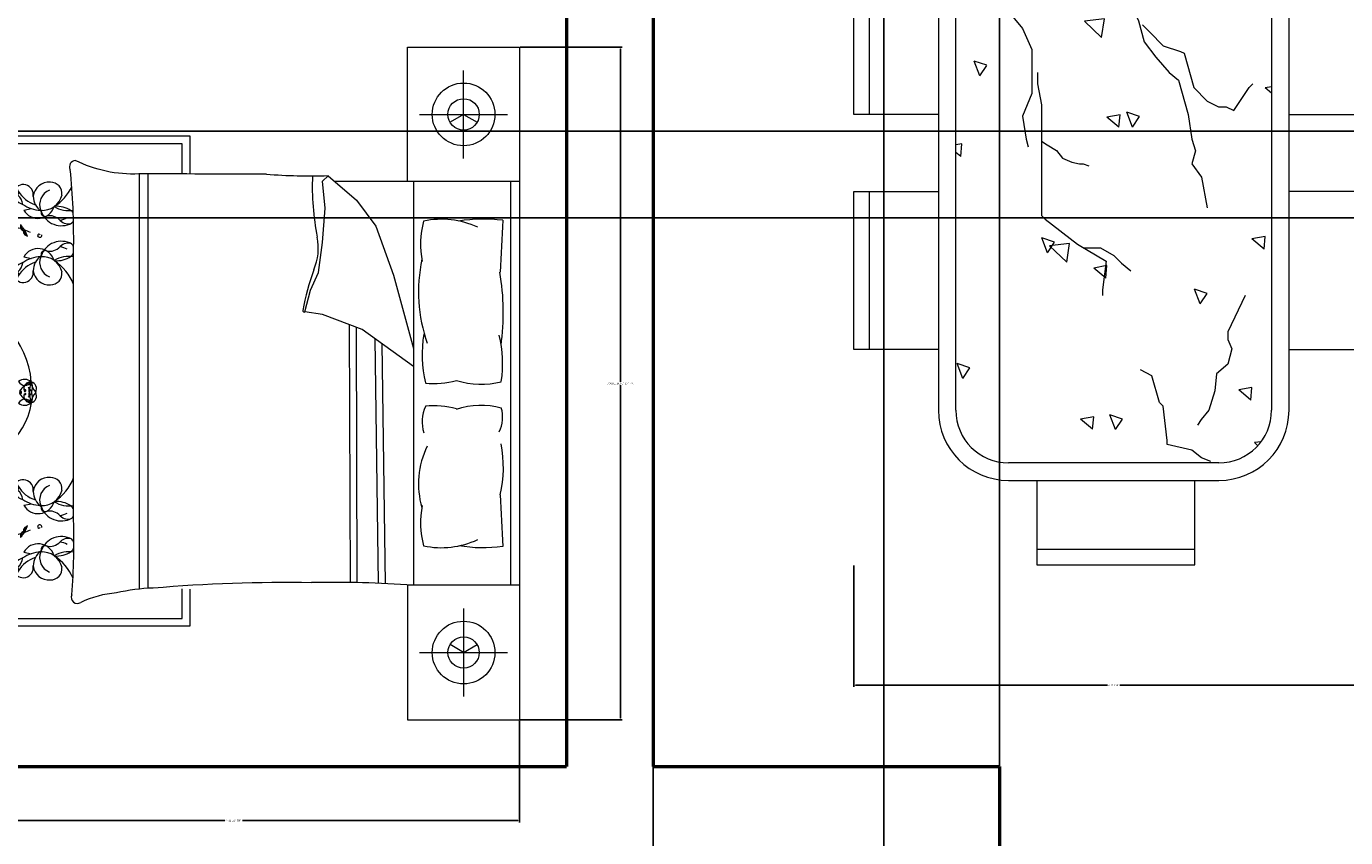
# Model space of a CAD drawing. Units: inches. Extents: x 3 to 576, y -689 to 51.
# Tile 7 of 21: x 199 to 336, y -514 to -429. Entities that reach past the tile are written whole.
import ezdxf

# ---------------------------------------------------------------- set-up
doc = ezdxf.new("R2010")
doc.units = ezdxf.units.IN
doc.header["$MEASUREMENT"] = 0
for name, color, linetype, lineweight in [('A-ANNO-DIMS', 2, 'Continuous', 18), ('A-FURN', 8, 'Continuous', 18), ('A-WALL', 7, 'Continuous', 50)]:
    doc.layers.add(name, color=color, linetype=linetype, lineweight=lineweight)
doc.styles.get("Standard").update_dxf_attribs({"font": 'arial.ttf'})
doc.dimstyles.get("Standard").update_dxf_attribs({"dimtxt": 0.18, "dimasz": 0.18, "dimexe": 0.18, "dimexo": 0.0625, "dimgap": 0.09, "dimtad": 0, "dimtih": 1, "dimtoh": 1, "dimdec": 0, "dimzin": 0, "dimdsep": 46, "dimlunit": 3, "dimtxsty": 'Standard', "dimcen": 0.09, "dimadec": 0, "dimazin": 0, "dimtfac": 1, "dimtdec": 0, "dimtofl": 0, "dimtmove": 0, "dimatfit": 3, "dimfxl": 1, "dimtolj": 1, "dimtzin": 0, "dimarcsym": 0})

# ---------------------------------------------------------------- blocks, each defined once
blk = doc.blocks.new('BED-DOUBLE')
for p, q in [((59.45, 69.91), (59.45, 0)), ((53.63, 58.35), (53.63, 67.49)), ((49.06, 62.92), (58.2, 62.92)), ((0, 60.68), (25.18, 60.68)), ((0, 9.72), (0, 60.68)), ((25.18, 60.68), (25.18, 56.73)), ((0.81, 59.87), (0.81, 10.53)), ((24.37, 59.87), (0.81, 59.87)), ((24.37, 56.73), (24.37, 59.87)), ((19.95, 13.6), (19.95, 56.73)), ((20.82, 13.66), (20.82, 56.73)), ((38.97, 55.99), (39.54, 56.55)), ((39.54, 56.55), (42.51, 54.01)), ((39.25, 53.16), (38.97, 55.99)), ((59.45, 55.93), (40.27, 55.93)), ((48.41, 55.93), (48.41, 13.98)), ((58.56, 13.98), (58.56, 55.93)), ((42.51, 54.01), (44.49, 51.31)), ((7.9, 52.98), (8.69, 53.14)), ((38.97, 49.62), (39.25, 53.16)), ((44.49, 51.31), (46.33, 46.22)), ((38.55, 46.5), (38.97, 49.62)), ((7.9, 48.1), (8.69, 47.94)), ((13.08, 20.76), (13.08, 49.15)), ((37.7, 44.66), (38.55, 46.5)), ((46.33, 46.22), (48.41, 38.59)), ((37.13, 42.39), (37.7, 44.66)), ((38.97, 42.11), (37.13, 42.39)), ((43.07, 40.55), (38.97, 42.11)), ((41.87, 14.23), (41.76, 41.05)), ((42.58, 14.23), (42.48, 40.78)), ((48.41, 36.72), (43.07, 40.55)), ((44.78, 14.2), (44.43, 39.58)), ((45.5, 14.17), (45.15, 39.06)), ((7.9, 22.3), (8.69, 22.46)), ((7.9, 17.41), (8.69, 17.26)), ((24.37, 10.53), (24.37, 13.61)), ((25.18, 13.59), (25.18, 9.72)), ((53.63, 11.56), (53.63, 2.42)), ((25.18, 9.72), (0, 9.72)), ((0.81, 10.53), (24.37, 10.53)), ((49.06, 6.99), (58.2, 6.99))]:
    blk.add_line(p, q)
for points in [[(47.8, 55.93), (47.8, 69.91), (59.45, 69.91)], [(53.63, 62.92), (52.22, 62.1)], [(53.63, 62.92), (55.04, 62.1)], [(59.45, 13.98), (47.8, 13.98), (47.8, 0), (59.45, 0)], [(53.63, 6.99), (52.22, 7.81)], [(53.63, 6.99), (55.04, 7.81)]]:
    blk.add_lwpolyline(points)
for points in [[(33.13, 56.7, 0.001242), (19.87, 56.73, -0.127202), (13.26, 58.14)], [(57.71, 51.91, 0.074897), (53.14, 51.83, -0.472817)], [(52.89, 35.28, 0.14099), (57.55, 35.14, 0.235245)], [(52.89, 32.3, -0.14099), (57.55, 32.44, -0.235245)], [(57.71, 18, -0.074897), (53.14, 18.08, 0.472817)], [(21.37, 13.68, 0.056112), (17.53, 13.18, 0.095341), (13.82, 12.19)]]:
    blk.add_lwpolyline(points, format="xyb")
for centre, radius in [((53.63, 62.92), 3.26), ((53.63, 62.92), 1.63), ((3.49, 50.11), 0.178), ((5.36, 48.94), 0.178), ((5.36, 21.45), 0.178), ((3.49, 20.29), 0.178), ((53.63, 6.99), 3.26), ((53.63, 6.99), 1.63)]:
    blk.add_circle(centre, radius)
for centre, radius, start, end in [((-2.47, 63.69), 5.54, 306.3036, 316.4814), ((-1.64, 62.09), 4.45, 303.4617, 330.1116), ((-0.42, 66.67), 9.13, 277.745, 311.8856), ((-1.32, 51.05), 9.13, 34.3865, 68.5908), ((13.3, 57.49), 0.645, 93.98, 207.3412), ((-0.61, 59.6), 3.71, 292.5547, 318.9546), ((1.38, 69.77), 12.63, 267.4081, 273.6519), ((-59.69, 49.98), 72.78, 359.3433, 5.6887), ((37.8, 120.65), 64.12, 265.8294, 271.553), ((64.29, 55.36), 26.39, 177.4519, 191.3392), ((6, 55.22), 1.01, 77.7115, 159.0387), ((5.45, 56.23), 0.762, 238.4633, 358.2869), ((7.95, 54.69), 2.31, 138.8402, 177.9352), ((6.56, 55.55), 0.747, 117.6827, 223.7762), ((6.09, 55.1), 0.0988, 223.7762, 159.7183), ((6.39, 55.47), 0.757, 2.9516, 103.728), ((12.45, 57.59), 6.39, 192.5173, 207.1824), ((5.37, 55.04), 1.44, 345.4653, 54.2343), ((7.54, 57.02), 1.56, 211.3827, 255.2969), ((7.84, 54.58), 1.05, 350.264, 160.8688), ((8.16, 54.83), 1.31, 175.969, 254.3045), ((6.7, 54.8), 0.643, 333.9755, 53.2681), ((10.15, 56.66), 3.3, 211.2614, 251.7045), ((10.53, 54.2), 1.67, 84.9449, 172.8857), ((11.17, 53.54), 1.62, 111.5819, 201.4221), ((10.7, 54.68), 1.18, 354.4856, 91.0538), ((8.16, 57.76), 5.29, 303.6671, 333.2997), ((5.76, 54.77), 0.113, 177.9352, 11.4834), ((5.81, 54.78), 0.0551, 11.4834, 127.9409), ((6.41, 53.42), 1.4, 6.1662, 51.5825), ((9.88, 56.69), 3.75, 236.2883, 266.5076), ((10.9, 54.49), 2.03, 182.3591, 234.0401), ((9.83, 55.04), 2.1, 265.2933, 346.921), ((5.91, 52.13), 0.137, 142.4737, 265.053), ((6.09, 52.15), 0.294, 127.7621, 169.0403), ((5.94, 52.4), 0.414, 265.053, 338.3618), ((6.48, 51.84), 0.541, 113.4276, 137.6104), ((6.42, 52.4), 0.178, 183.2768, 356.7232), ((6.55, 52.07), 0.291, 139.7889, 227.6792), ((5.87, 52.08), 0.583, 353.0852, 15.7171), ((6.25, 52.01), 0.368, 350.3487, 43.6538), ((6.93, 52.39), 0.428, 198.7263, 262.5032), ((6.59, 52.19), 0.17, 1.1081, 91.8675), ((6.91, 52.1), 0.138, 255.2356, 54.9248), ((6.7, 52.15), 0.297, 11.5637, 52.6358), ((9.4, 53.85), 1.74, 209.9085, 343.1337), ((10.13, 52.75), 0.434, 167.3041, 285.1471), ((11.31, 50.67), 2.7, 122.7011, 126.3445), ((11.81, 53.58), 2.23, 199.2822, 299.1751), ((10.62, 50.95), 1.43, 41.5653, 105.1471), ((12.57, 55.82), 2.9, 238.8218, 279.1554), ((11.31, 50.67), 2.7, 55.785, 94.7304), ((11.41, 53.92), 2.01, 277.436, 299.9149), ((12.31, 52.24), 0.842, 30.0293, 52.325), ((3.75, 51.26), 0.199, 124.3538, 214.3923), ((4.04, 51.23), 0.464, 190.3057, 287.1958), ((4.17, 51.39), 0.538, 176.9701, 248.2913), ((8.01, 54.23), 5.2, 212.6784, 216.3746), ((3.99, 51.27), 0.206, 216.3746, 291.7548), ((5.81, 48.38), 2.9, 124.0033, 132.4917), ((2.83, 48.01), 3.1, 63.7819, 68.2913), ((4.48, 50.4), 0.493, 128.3208, 208.8162), ((4.48, 51.12), 0.464, 122.8155, 187.3992), ((4.12, 50.93), 0.155, 289.3605, 111.7548), ((4.24, 50.93), 0.155, 221.8703, 44.2646), ((4.94, 50.48), 0.812, 157.2305, 229.0635), ((4.69, 51.06), 0.538, 109.4799, 177.6828), ((4.67, 50.75), 0.478, 174.4544, 220.6188), ((4.4, 51.4), 0.199, 56.8636, 146.9021), ((4.5, 51.18), 0.206, 148.8844, 224.2646), ((8.78, 48.6), 5.2, 145.1882, 148.8844), ((5.81, 48.38), 2.9, 94.756, 119.2041), ((11.99, 44.2), 9.55, 132.2412, 142.1744), ((7.17, 51.8), 1.97, 178.3264, 187.1302), ((5.04, 51.53), 0.367, 11.3256, 64.4621), ((6.29, 52.06), 1.1, 190.2588, 210.656), ((5.55, 51.61), 0.336, 188.3432, 274.2869), ((5.84, 51.79), 0.586, 210.656, 242.6341), ((6.28, 52.3), 1.12, 218.2101, 226.3071), ((5.45, 51.35), 0.142, 325.7657, 67.4417), ((1.03, 56.11), 6.64, 313.1541, 322.0459), ((5.96, 45.49), 5.79, 73.5842, 93.8277), ((6.46, 51.97), 0.153, 227.6792, 350.3487), ((9.52, 51.39), 1.97, 178.3264, 187.1302), ((7.39, 51.11), 0.367, 11.3256, 64.4621), ((8.64, 51.64), 1.1, 190.2588, 210.656), ((7.9, 51.19), 0.336, 188.3432, 274.2869), ((8.19, 51.38), 0.586, 210.656, 242.6341), ((8.64, 51.88), 1.12, 218.2101, 226.3071), ((7.81, 50.93), 0.142, 325.7657, 67.4417), ((8.21, 50.67), 0.336, 147.5332, 233.4768), ((7.94, 50.71), 0.142, 354.3784, 96.0543), ((8.51, 50.85), 0.586, 179.1859, 211.164), ((5.96, 45.49), 5.79, 63.0032, 69.8941), ((12.48, 52.59), 1.05, 221.5653, 293.8354), ((12.31, 52.24), 0.842, 314.4517, 333.558), ((58.53, 49.42), 9.37, 165.1039, 191.0369), ((51.31, 43.01), 9.01, 65.1316, 101.7583), ((723.03, 13.38), 666.43, 176.68521, 177.14978), ((2.98, 49.84), 0.137, 142.4737, 265.053), ((3.16, 49.87), 0.294, 61.2196, 169.0403), ((3, 50.12), 0.414, 265.053, 338.3618), ((3.35, 50.47), 0.351, 157.4086, 261.4386), ((3.15, 50.48), 0.176, 58.0499, 135.6268), ((3.55, 49.55), 0.541, 113.4276, 137.6104), ((3.34, 50.37), 0.118, 172.906, 277.132), ((2.95, 50.16), 0.561, 14.7558, 58.0499), ((3.62, 49.79), 0.291, 139.7889, 227.6792), ((3.53, 49.68), 0.153, 227.6792, 350.3487), ((3.74, 50.31), 0.243, 36.1046, 181.4281), ((2.93, 49.79), 0.583, 353.0852, 15.7171), ((3.31, 49.72), 0.368, 350.3487, 43.6538), ((3.59, 50.5), 0.245, 270.0645, 331.1507), ((3.8, 50.44), 0.28, 221.8413, 265.7877), ((4, 50.1), 0.428, 198.7263, 262.5032), ((3.66, 49.9), 0.17, 1.1081, 91.8675), ((3.8, 50.33), 0.174, 263.7526, 41.7054), ((3.76, 49.86), 0.297, 11.5637, 86.365), ((3.98, 49.81), 0.138, 255.2356, 54.9248), ((4.57, 50.43), 0.59, 207.7043, 254.3516), ((4.19, 50.1), 0.812, 270.278, 342.111), ((4.73, 49.08), 0.574, 98.7227, 159.3375), ((1.96, 48.08), 3.48, 30.544, 49.818), ((3.87, 50.06), 0.574, 340.0041, 40.6188), ((4.57, 50.12), 0.478, 278.7227, 324.8872), ((4.49, 49.73), 0.493, 290.5253, 358.5375), ((5.23, 49.31), 0.351, 157.4086, 261.4386), ((5.03, 49.32), 0.176, 58.0499, 135.6268), ((5.45, 49.87), 0.493, 182.8499, 266.1226), ((5.26, 50.22), 0.478, 231.7607, 277.9252), ((5.63, 50.31), 0.812, 214.5369, 286.3699), ((4.83, 48.99), 0.561, 14.7558, 58.0499), ((1.96, 48.08), 3.48, 23.0501, 23.8477), ((5.4, 49.18), 0.574, 37.3105, 97.9252), ((5.61, 49.14), 0.243, 36.1046, 181.4281), ((5.47, 49.97), 0.59, 265.0106, 311.658), ((8.95, 51.12), 1.1, 211.164, 231.5612), ((9.15, 52.01), 1.97, 234.6898, 243.4936), ((9.16, 51), 1.12, 195.5129, 203.6099), ((7.9, 50.27), 0.367, 357.3579, 50.4944), ((9.48, 50.34), 0.135, 12.7051, 190.4384), ((9.56, 50.36), 0.219, 190.4384, 10.4136), ((11.81, 47.5), 2.23, 60.8249, 160.7178), ((12.48, 48.49), 1.05, 66.1646, 138.4347), ((12.31, 48.84), 0.842, 23.229, 45.5483), ((32.84, 49.05), 5.69, 336.2616, 11.3392), ((4.44, 49.82), 0.59, 244.9899, 291.6373), ((4.85, 48.67), 0.137, 142.4737, 265.053), ((5.03, 48.7), 0.294, 61.2196, 169.0403), ((4.88, 48.95), 0.414, 265.053, 338.3618), ((5.43, 48.38), 0.541, 113.4276, 137.6104), ((5.21, 49.21), 0.118, 172.906, 277.132), ((5.5, 48.62), 0.291, 139.7889, 227.6792), ((5.4, 48.52), 0.153, 227.6792, 350.3487), ((4.81, 48.63), 0.583, 353.0852, 15.7171), ((1.96, 48.08), 3.48, 357.1071, 4.7585), ((5.19, 48.56), 0.368, 350.3487, 43.6538), ((5.47, 49.33), 0.245, 270.0645, 331.1507), ((5.68, 49.27), 0.28, 221.8413, 265.7877), ((5.87, 48.94), 0.428, 198.7263, 262.5032), ((5.53, 48.74), 0.17, 1.1081, 91.8675), ((5.68, 49.17), 0.174, 263.7526, 41.7054), ((5.64, 48.7), 0.297, 11.5637, 86.365), ((5.85, 48.65), 0.138, 255.2356, 54.9248), ((9.88, 44.39), 3.75, 93.4924, 123.7117), ((9.4, 47.23), 1.74, 16.8663, 150.0915), ((10.9, 46.59), 2.03, 125.9599, 177.6409), ((11.17, 47.54), 1.62, 158.5779, 248.4181), ((9.83, 46.04), 2.1, 13.079, 94.7067), ((10.13, 48.33), 0.434, 74.8529, 192.6959), ((11.31, 50.41), 2.7, 233.6555, 237.2989), ((10.62, 50.13), 1.43, 254.8529, 318.4347), ((12.57, 45.26), 2.9, 79.7133, 121.1782), ((11.31, 50.41), 2.7, 265.2696, 304.215), ((11.41, 47.16), 2.01, 60.0851, 82.564), ((12.31, 48.84), 0.842, 307.675, 336.7144), ((8.16, 46.25), 1.31, 105.6955, 184.031), ((7.84, 46.5), 1.05, 199.1312, 9.736), ((6.41, 47.66), 1.4, 308.4175, 353.8338), ((10.15, 44.42), 3.3, 108.2955, 148.7386), ((10.53, 46.88), 1.67, 187.1143, 275.0551), ((8.16, 43.32), 5.29, 21.4941, 56.3329), ((63.55, 37.54), 27.11, 160.1194, 169.3383), ((65.19, 44.49), 16.25, 168.0397, 199.2615), ((5.45, 44.85), 0.762, 1.7131, 121.5367), ((6, 45.86), 1.01, 200.9613, 282.2885), ((5.76, 46.31), 0.113, 348.5166, 182.0648), ((7.95, 46.39), 2.31, 182.0648, 221.1598), ((5.81, 46.3), 0.0551, 232.0591, 348.5166), ((6.56, 45.54), 0.747, 136.2238, 242.3173), ((6.13, 45.97), 0.0595, 200.2667, 136.2271), ((5.37, 46.05), 1.44, 305.7657, 14.5347), ((12.45, 43.49), 6.39, 152.8176, 167.4827), ((6.39, 45.61), 0.757, 256.272, 357.0484), ((7.54, 44.06), 1.56, 104.7031, 148.6173), ((6.7, 46.28), 0.643, 306.7319, 26.0245), ((10.7, 46.4), 1.18, 268.9462, 5.5144), ((32.41, 42.33), 25.35, 352.2196, 9.497), ((-0.61, 41.48), 3.71, 41.0454, 67.4453), ((1.38, 31.32), 12.63, 86.3481, 92.5919), ((-1.32, 50.03), 9.13, 291.4092, 325.6135), ((-0.42, 34.41), 9.13, 4.4623, 82.255), ((-1.64, 38.99), 4.45, 1.272, 56.5383), ((37.07, 42.55), 0.169, 178.8623, 289.7536), ((-2.47, 37.39), 5.54, 17.8504, 53.6964), ((-4.03, 34.48), 8.25, 34.0123, 54.053), ((61.64, 37.91), 12.33, 169.8617, 193.6238), ((45.23, 36.98), 12.46, 351.5249, 13.96), ((-3.99, 37.66), 5.02, 343.5431, 17.0202), ((-5.31, 35.11), 9.13, 4.4623, 27.4146), ((-6.58, 35.67), 7.42, 4.3787, 5.6357), ((-11.66, 31.77), 13.27, 19.7217, 19.9028), ((3.11, 35.07), 1.01, 47.7873, 129.1145), ((3.14, 36.22), 0.762, 208.5391, 328.3627), ((4.54, 33.64), 2.31, 108.9159, 148.011), ((3.76, 35.07), 0.747, 87.7585, 193.852), ((9.89, 33.91), 6.39, 162.593, 177.2582), ((2.48, 35.23), 1.44, 315.5411, 24.3101), ((5.35, 35.86), 1.56, 181.4585, 225.3727), ((3.58, 35.09), 0.757, 333.0274, 73.8037), ((2.68, 34.8), 0.113, 148.011, 341.5592), ((2.73, 34.78), 0.0551, 341.5592, 98.0167), ((3.13, 34.92), 0.0988, 193.852, 129.9245), ((8, 34.37), 1.01, 47.7873, 129.1145), ((8.03, 35.52), 0.762, 208.5391, 328.3627), ((9.43, 32.94), 2.31, 108.9159, 148.011), ((8.65, 34.38), 0.747, 87.7585, 193.852), ((8.02, 34.22), 0.0988, 193.852, 129.9245), ((7.37, 34.53), 1.44, 315.5411, 24.3101), ((14.78, 33.21), 6.39, 162.593, 177.2582), ((7.37, 33.54), 1.44, 335.6899, 44.4589), ((14.78, 34.86), 6.39, 182.7418, 197.407), ((8.47, 34.4), 0.757, 333.0274, 73.8037), ((10.24, 35.16), 1.56, 181.4585, 225.3727), ((50.55, 43.52), 8.57, 264.0129, 285.8293), ((1.69, 33.95), 7.07, 262.8636, 351.8197), ((2.68, 33.27), 0.113, 18.4408, 211.989), ((4.54, 34.43), 2.31, 211.989, 251.0841), ((2.73, 33.29), 0.0551, 261.9833, 18.4408), ((3.76, 32.99), 0.747, 166.148, 272.2415), ((3.17, 33.16), 0.0595, 230.1909, 166.0209), ((9.89, 34.16), 6.39, 182.7418, 197.407), ((2.48, 32.84), 1.44, 335.6899, 44.4589), ((5.35, 32.21), 1.56, 134.6273, 178.5415), ((3.58, 32.97), 0.757, 286.1963, 26.9726), ((8.03, 32.55), 0.762, 31.6373, 151.4609), ((8, 33.7), 1.01, 230.8855, 312.2127), ((7.57, 34.1), 0.113, 148.011, 341.5592), ((7.57, 33.97), 0.113, 18.4408, 211.989), ((9.43, 35.13), 2.31, 211.989, 251.0841), ((7.62, 34.08), 0.0551, 341.5592, 98.0167), ((7.62, 33.99), 0.0551, 261.9833, 18.4408), ((8.65, 33.69), 0.747, 166.148, 272.2415), ((8.06, 33.86), 0.0595, 230.1909, 166.0209), ((8.47, 33.67), 0.757, 286.1963, 26.9726), ((10.24, 32.91), 1.56, 134.6273, 178.5415), ((-3.99, 30.4), 5.02, 342.9798, 16.4569), ((-6.58, 32.39), 7.42, 354.3643, 355.6213), ((-11.66, 36.3), 13.27, 340.0972, 340.2783), ((3.14, 31.85), 0.762, 31.6373, 151.4609), ((3.11, 33), 1.01, 230.8855, 312.2127), ((-5.31, 32.96), 9.13, 332.5854, 355.5377), ((53.02, 31.01), 3.71, 155.0183, 198.5407), ((50.55, 24.06), 8.57, 74.1707, 95.9871), ((54.23, 31.48), 3.46, 333.3437, 16.1026), ((2.33, 33.04), 4.09, 248.117, 276.6195), ((1.2, 29.29), 1.64, 256.3898, 349.0739), ((1.42, 30.52), 2.07, 252.8609, 311.9049), ((-1.32, 20.37), 9.13, 34.3865, 68.5908), ((57.84, 24.53), 8.9, 153.8761, 196.1746), ((45.48, 26.29), 12.29, 346.3427, 11.1841), ((1.38, 39.08), 12.63, 267.4081, 273.6519), ((-0.61, 28.92), 3.71, 292.5547, 318.9546), ((6, 24.53), 1.01, 77.7115, 159.0387), ((5.45, 25.55), 0.762, 238.4633, 358.2869), ((7.95, 24), 2.31, 138.8402, 177.9352), ((6.56, 24.86), 0.747, 117.6827, 223.7762), ((6.39, 24.79), 0.757, 2.9516, 103.728), ((7.54, 26.34), 1.56, 211.3827, 255.2969), ((5.37, 24.35), 1.44, 345.4653, 54.2343), ((12.45, 26.91), 6.39, 192.5173, 207.1824), ((7.84, 23.9), 1.05, 350.264, 160.8688), ((10.53, 23.52), 1.67, 84.9449, 172.8857), ((10.7, 24), 1.18, 354.4856, 91.0538), ((8.16, 27.08), 5.29, 303.6671, 338.5059), ((5.76, 24.08), 0.113, 177.9352, 11.4834), ((5.81, 24.09), 0.0551, 11.4834, 127.9409), ((6.09, 24.41), 0.0988, 223.7762, 159.7183), ((8.16, 24.15), 1.31, 175.969, 254.3045), ((6.7, 24.12), 0.643, 333.9755, 53.2681), ((6.41, 22.74), 1.4, 6.1662, 51.5825), ((10.15, 25.98), 3.3, 211.2614, 251.7045), ((10.9, 23.81), 2.03, 182.3591, 234.0401), ((11.17, 22.86), 1.62, 111.5819, 201.4221), ((9.83, 24.36), 2.1, 265.2933, 346.921), ((723.03, 56.53), 666.43, 182.85022, 183.31479), ((5.5, 21.78), 0.291, 132.3208, 220.2111), ((5.4, 21.88), 0.153, 9.6513, 132.3208), ((1.96, 22.32), 3.48, 355.2415, 2.8929), ((9.88, 26.01), 3.75, 236.2883, 266.5076), ((9.4, 23.17), 1.74, 209.9085, 343.1337), ((10.13, 22.07), 0.434, 167.3041, 285.1471), ((11.31, 19.99), 2.7, 122.7011, 126.3445), ((11.81, 22.9), 2.23, 199.2822, 299.1751), ((12.57, 25.14), 2.9, 238.8218, 280.2867), ((11.31, 19.99), 2.7, 55.785, 94.7304), ((12.31, 21.55), 0.842, 23.2856, 52.325), ((58.53, 20.49), 9.37, 168.9631, 194.8961), ((2.98, 20.56), 0.137, 94.947, 217.5263), ((3, 20.28), 0.414, 21.6382, 94.947), ((3.62, 20.61), 0.291, 132.3208, 220.2111), ((3.53, 20.71), 0.153, 9.6513, 132.3208), ((2.93, 20.61), 0.583, 344.2829, 6.9148), ((3.31, 20.68), 0.368, 316.3462, 9.6513), ((4, 20.3), 0.428, 97.4968, 161.2737), ((3.98, 20.59), 0.138, 305.0752, 104.7644), ((4.44, 20.58), 0.59, 68.3627, 115.0101), ((4.19, 20.3), 0.812, 17.889, 89.722), ((4.73, 21.32), 0.574, 200.6625, 261.2773), ((4.57, 20.28), 0.478, 35.1128, 81.2773), ((4.49, 20.66), 0.493, 1.4625, 69.4747), ((4.85, 21.72), 0.137, 94.947, 217.5263), ((5.03, 21.7), 0.294, 190.9597, 298.7804), ((4.88, 21.45), 0.414, 21.6382, 94.947), ((5.23, 21.09), 0.351, 98.5614, 202.5914), ((5.03, 21.08), 0.176, 224.3732, 301.9501), ((5.45, 20.52), 0.493, 93.8774, 177.1501), ((5.63, 20.09), 0.812, 73.6301, 145.4631), ((5.26, 20.18), 0.478, 82.0748, 128.2393), ((5.43, 22.01), 0.541, 222.3896, 246.5724), ((5.21, 21.19), 0.118, 82.868, 187.094), ((4.83, 21.41), 0.561, 301.9501, 345.2442), ((1.96, 22.32), 3.48, 336.1523, 336.9499), ((5.4, 21.22), 0.574, 262.0748, 322.6895), ((4.81, 21.77), 0.583, 344.2829, 6.9148), ((5.61, 21.26), 0.243, 178.5719, 323.8954), ((5.47, 20.43), 0.59, 48.342, 94.9894), ((5.19, 21.84), 0.368, 316.3462, 9.6513), ((5.87, 21.46), 0.428, 97.4968, 161.2737), ((5.68, 21.12), 0.28, 94.2123, 138.1587), ((5.47, 21.07), 0.245, 28.8493, 89.9355), ((5.53, 21.66), 0.17, 268.1325, 358.8919), ((5.64, 21.7), 0.297, 273.635, 348.4363), ((5.68, 21.23), 0.174, 318.2946, 96.2474), ((5.85, 21.75), 0.138, 305.0752, 104.7644), ((10.62, 20.26), 1.43, 41.5653, 105.1471), ((11.41, 23.23), 2.01, 277.436, 299.9149), ((12.48, 21.91), 1.05, 221.5653, 293.8354), ((-54.91, 18.62), 68.03, 355.2402, 1.8035), ((12.31, 21.55), 0.842, 314.4517, 336.7144), ((3.16, 20.53), 0.294, 190.9597, 298.7804), ((3.35, 19.93), 0.351, 98.5614, 202.5914), ((3.15, 19.91), 0.176, 224.3732, 301.9501), ((3.55, 20.85), 0.541, 222.3896, 246.5724), ((3.34, 20.03), 0.118, 82.868, 187.094), ((2.95, 20.24), 0.561, 301.9501, 345.2442), ((3.74, 20.09), 0.243, 178.5719, 323.8954), ((3.75, 19.14), 0.199, 145.6077, 235.6462), ((4.04, 19.17), 0.464, 72.8042, 169.6943), ((3.8, 19.96), 0.28, 94.2123, 138.1587), ((3.59, 19.9), 0.245, 28.8493, 89.9355), ((4.17, 19.01), 0.538, 111.7087, 183.0299), ((8.01, 16.17), 5.2, 143.6254, 147.3216), ((3.66, 20.5), 0.17, 268.1325, 358.8919), ((3.76, 20.54), 0.297, 273.635, 348.4363), ((3.8, 20.07), 0.174, 318.2946, 96.2474), ((3.99, 19.13), 0.206, 68.2452, 143.6254), ((5.81, 22.02), 2.9, 227.5083, 235.9967), ((2.83, 22.39), 3.1, 291.7087, 296.2181), ((4.48, 20), 0.493, 151.1838, 231.6792), ((4.48, 19.27), 0.464, 172.6008, 237.1845), ((4.57, 19.96), 0.59, 105.6484, 152.2957), ((4.12, 19.47), 0.155, 248.2452, 70.6395), ((4.94, 19.92), 0.812, 130.9365, 202.7695), ((4.24, 19.47), 0.155, 315.7354, 138.1297), ((4.69, 19.33), 0.538, 182.3172, 250.5201), ((4.67, 19.65), 0.478, 139.3812, 185.5456), ((1.96, 22.32), 3.48, 310.182, 329.456), ((4.5, 19.21), 0.206, 135.7354, 211.1156), ((3.87, 20.33), 0.574, 319.3812, 19.9959), ((5.81, 22.02), 2.9, 240.7959, 265.244), ((11.99, 26.2), 9.55, 217.8256, 227.7588), ((5.96, 24.9), 5.79, 266.1723, 286.4158), ((8.64, 18.76), 1.1, 149.344, 169.7412), ((9.52, 19.01), 1.97, 172.8698, 181.6736), ((7.39, 19.29), 0.367, 295.5379, 348.6744), ((7.9, 19.21), 0.336, 85.7131, 171.6568), ((8.19, 19.02), 0.586, 117.3659, 149.344), ((8.64, 18.52), 1.12, 133.6929, 141.7899), ((7.81, 19.46), 0.142, 292.5583, 34.2343), ((8.21, 19.72), 0.336, 126.5232, 212.4668), ((8.51, 19.55), 0.586, 148.836, 180.8141), ((7.94, 19.68), 0.142, 263.9457, 5.6216), ((5.96, 24.9), 5.79, 290.1059, 296.9968), ((8.95, 19.28), 1.1, 128.4388, 148.836), ((9.15, 18.38), 1.97, 116.5064, 125.3102), ((9.16, 19.4), 1.12, 156.3901, 164.4871), ((7.9, 20.13), 0.367, 309.5056, 2.6421), ((9.56, 20.04), 0.219, 349.5864, 169.5616), ((9.48, 20.06), 0.135, 169.5616, 347.2949), ((4.4, 18.99), 0.199, 213.0979, 303.1364), ((8.78, 21.8), 5.2, 211.1156, 214.8118), ((6.29, 18.34), 1.1, 149.344, 169.7412), ((7.17, 18.6), 1.97, 172.8698, 181.6736), ((5.04, 18.87), 0.367, 295.5379, 348.6744), ((5.55, 18.79), 0.336, 85.7131, 171.6568), ((5.84, 18.61), 0.586, 117.3659, 149.344), ((6.28, 18.1), 1.12, 133.6929, 141.7899), ((5.45, 19.05), 0.142, 292.5583, 34.2343), ((1.03, 14.28), 6.64, 37.9541, 46.8459), ((5.91, 18.27), 0.137, 94.947, 217.5263), ((6.09, 18.24), 0.294, 190.9597, 232.2379), ((5.94, 18), 0.414, 21.6382, 94.947), ((6.48, 18.56), 0.541, 222.3896, 246.5724), ((6.42, 18), 0.178, 3.2768, 176.7232), ((6.55, 18.32), 0.291, 132.3208, 220.2111), ((6.46, 18.43), 0.153, 9.6513, 132.3208), ((5.87, 18.32), 0.583, 344.2829, 6.9148), ((6.25, 18.39), 0.368, 316.3462, 9.6513), ((6.93, 18.01), 0.428, 97.4968, 161.2737), ((6.59, 18.21), 0.17, 268.1325, 358.8919), ((6.91, 18.3), 0.138, 305.0752, 104.7644), ((6.7, 18.25), 0.297, 307.3642, 348.4363), ((9.4, 16.55), 1.74, 16.8663, 150.0915), ((10.13, 17.65), 0.434, 74.8529, 192.6959), ((11.81, 16.82), 2.23, 60.8249, 160.7178), ((10.62, 19.45), 1.43, 254.8529, 318.4347), ((11.41, 16.48), 2.01, 60.0851, 82.564), ((12.48, 17.81), 1.05, 66.1646, 138.4347), ((12.31, 18.16), 0.842, 307.675, 342.5814), ((12.31, 18.16), 0.842, 16.6343, 45.5483), ((51.31, 26.9), 9.01, 258.2417, 294.8684), ((8.16, 15.56), 1.31, 105.6955, 184.031), ((6.41, 16.98), 1.4, 308.4175, 353.8338), ((10.15, 13.74), 3.3, 108.2955, 148.7386), ((9.88, 13.7), 3.75, 93.4924, 123.7117), ((10.9, 15.91), 2.03, 125.9599, 177.6409), ((11.17, 16.86), 1.62, 158.5779, 248.4181), ((9.83, 15.35), 2.1, 13.079, 94.7067), ((11.31, 19.72), 2.7, 233.6555, 237.2989), ((12.57, 14.57), 2.9, 79.249, 121.1782), ((11.31, 19.72), 2.7, 265.2696, 304.215), ((8.16, 12.63), 5.29, 23.6453, 56.3329), ((5.76, 15.63), 0.113, 348.5166, 182.0648), ((7.95, 15.71), 2.31, 182.0648, 221.1598), ((5.81, 15.62), 0.0551, 232.0591, 348.5166), ((6.56, 14.85), 0.747, 136.2238, 242.3173), ((6.13, 15.29), 0.0595, 200.2667, 136.2271), ((12.45, 12.81), 6.39, 152.8176, 167.4827), ((5.37, 15.36), 1.44, 305.7657, 14.5347), ((7.84, 15.82), 1.05, 199.1312, 9.736), ((6.7, 15.6), 0.643, 306.7319, 26.0245), ((10.53, 16.2), 1.67, 187.1143, 275.0551), ((10.7, 15.72), 1.18, 268.9462, 5.5144), ((-0.61, 10.8), 3.71, 41.0454, 67.4453), ((-1.32, 19.35), 9.13, 291.4092, 325.6135), ((5.45, 14.17), 0.762, 1.7131, 121.5367), ((6, 15.18), 1.01, 200.9613, 282.2885), ((7.54, 13.38), 1.56, 104.7031, 148.6173), ((6.39, 14.93), 0.757, 256.272, 357.0484), ((35.29, -149.59), 163.86, 89.1145, 94.8735), ((39.86, -111.34), 125.62, 86.1, 90.9282), ((1.38, 0.63), 12.63, 86.3481, 92.5919), ((-0.42, 3.73), 9.13, 48.1144, 82.255), ((13.47, 12.72), 0.637, 156.5219, 303.8264), ((-1.64, 8.31), 4.45, 29.8884, 56.5383), ((-2.47, 6.71), 5.54, 43.5186, 53.6964)]:
    blk.add_arc(centre, radius, start, end)
blk = doc.blocks.new('DINING-SET-6')
for p, q in [((35.44, 83.21), (19.03, 83.21)), ((19.03, 83.21), (19.03, 74.43)), ((35.44, 74.43), (35.44, 83.21)), ((19.03, 81.61), (35.44, 81.61)), ((37.96, 74.43), (16.08, 74.43)), ((16.08, 72.6), (37.96, 72.6)), ((8.79, 67.13), (8.79, 16.08)), ((10.61, 16.08), (10.61, 67.13)), ((20.49, 66.46), (21.48, 64.87)), ((43.43, 67.13), (43.43, 16.08)), ((45.25, 16.08), (45.25, 67.13)), ((21.9, 63.9), (21.31, 65.43)), ((22.64, 64.98), (21.31, 65.43)), ((21.48, 64.87), (23.07, 63.29)), ((21.9, 63.9), (22.63, 64.98)), ((0, 46.82), (0, 63.23)), ((0, 63.23), (8.79, 63.23)), ((1.6, 63.23), (1.6, 46.82)), ((12.38, 64.08), (12.77, 63.09)), ((23.07, 63.29), (24.85, 62.49)), ((54.04, 63.23), (45.25, 63.23)), ((52.44, 63.23), (52.44, 46.82)), ((54.04, 46.82), (54.04, 63.23)), ((12.77, 63.09), (14.75, 59.12)), ((24.85, 62.49), (25.84, 62.3)), ((25.84, 62.3), (26.44, 61.7)), ((29.06, 62.49), (27.69, 62.24)), ((28.94, 61.18), (27.69, 62.24)), ((28.94, 61.18), (29.06, 62.49)), ((26.44, 61.7), (27.43, 60.91)), ((27.43, 60.91), (28.22, 59.52)), ((12.6, 59.46), (11.23, 59.2)), ((12.49, 58.15), (11.23, 59.2)), ((12.49, 58.15), (12.6, 59.46)), ((14.75, 59.12), (17.52, 55.75)), ((28.22, 59.52), (29.6, 56.55)), ((38.5, 59.66), (37.18, 60.1)), ((37.77, 58.57), (37.18, 60.1)), ((37.77, 58.57), (38.5, 59.66)), ((26.06, 56.77), (23.98, 56.52)), ((25.76, 54.82), (23.98, 56.52)), ((25.76, 54.82), (26.06, 56.77)), ((29.6, 56.55), (30.2, 54.36)), ((17.52, 55.75), (18.51, 53.57)), ((30, 56.15), (30.79, 55.36)), ((30.79, 55.36), (32.18, 53.97)), ((18.51, 53.57), (18.51, 49.01)), ((30.2, 54.36), (31.39, 52.78)), ((32.18, 53.97), (33.96, 53.37)), ((13.09, 50.84), (12.5, 52.37)), ((13.83, 51.93), (12.5, 52.37)), ((31.39, 52.78), (32.77, 51.19)), ((33.96, 53.37), (34.36, 53.18)), ((34.36, 53.18), (35.35, 49.61)), ((13.09, 50.84), (13.83, 51.92)), ((19.11, 51.19), (19.11, 50)), ((32.77, 51.19), (33.76, 50.4)), ((19.11, 50), (19.5, 47.82)), ((33.76, 50.4), (34.75, 46.83)), ((35.35, 49.61), (36.73, 48.22)), ((39.5, 47.23), (41.09, 49.61)), ((41.09, 49.61), (41.49, 50)), ((43.43, 49.7), (42.77, 49.58)), ((43.43, 49.03), (42.77, 49.58)), ((18.51, 49.01), (17.52, 46.63)), ((36.73, 48.22), (37.92, 47.62)), ((8.79, 46.82), (0, 46.82)), ((19.5, 47.82), (19.5, 36.32)), ((27.69, 46.8), (26.31, 46.55)), ((27.57, 45.49), (27.68, 46.8)), ((28.96, 45.51), (28.37, 47.05)), ((29.69, 46.6), (28.37, 47.05)), ((34.75, 46.83), (35.15, 44.25)), ((37.92, 47.62), (38.71, 47.62)), ((38.71, 47.62), (39.5, 47.23)), ((45.25, 46.82), (54.04, 46.82)), ((17.52, 46.63), (17.92, 44.25)), ((27.57, 45.49), (26.31, 46.55)), ((28.96, 45.51), (29.69, 46.6)), ((17.92, 44.25), (18.12, 43.46)), ((19.5, 44.06), (20.09, 43.66)), ((35.15, 44.25), (35.54, 43.06)), ((11.23, 43.76), (10.61, 43.65)), ((11.11, 42.46), (10.61, 42.88)), ((11.11, 42.46), (11.23, 43.76)), ((20.09, 43.66), (21.08, 43.07)), ((21.08, 43.07), (21.68, 42.27)), ((35.54, 43.06), (35.15, 41.68)), ((21.68, 42.27), (22.67, 41.88)), ((22.67, 41.88), (23.46, 41.68)), ((23.46, 41.68), (23.85, 41.68)), ((23.85, 41.68), (24.45, 41.48)), ((35.15, 41.68), (36.14, 40.29)), ((36.14, 40.29), (36.73, 37.12)), ((0, 22.39), (0, 38.8)), ((0, 38.8), (8.79, 38.8)), ((1.6, 38.8), (1.6, 22.39)), ((54.04, 38.8), (45.25, 38.8)), ((52.44, 38.8), (52.44, 22.39)), ((54.04, 22.39), (54.04, 38.8)), ((19.5, 36.32), (19.9, 35.93)), ((19.9, 35.93), (23.27, 33.35)), ((20.15, 32.45), (19.56, 33.99)), ((20.88, 33.54), (19.56, 33.99)), ((20.15, 32.45), (20.88, 33.54)), ((22.44, 33.42), (20.36, 33.17)), ((22.14, 31.47), (20.36, 33.17)), ((22.14, 31.47), (22.44, 33.42)), ((23.27, 33.35), (26.24, 31.57)), ((23.86, 32.95), (25.64, 32.95)), ((25.64, 32.95), (27.03, 32.16)), ((42.77, 34.14), (41.4, 33.89)), ((42.65, 32.83), (41.4, 33.89)), ((42.65, 32.83), (42.77, 34.14)), ((26.24, 31.57), (25.84, 28.59)), ((27.03, 32.16), (27.82, 31.37)), ((26.31, 31.11), (24.94, 30.85)), ((26.2, 29.8), (24.94, 30.85)), ((26.2, 29.8), (26.31, 31.11)), ((27.82, 31.37), (28.81, 30.57)), ((25.84, 28.59), (25.84, 28)), ((36.01, 27.13), (35.43, 28.66)), ((36.75, 28.22), (35.43, 28.66)), ((36.01, 27.13), (36.75, 28.22)), ((40.69, 28), (38.9, 24.23)), ((38.9, 24.23), (38.9, 23.44)), ((38.9, 23.44), (39.3, 22.45)), ((8.79, 22.39), (0, 22.39)), ((39.3, 22.45), (38.9, 20.86)), ((45.25, 22.39), (54.04, 22.39)), ((11.34, 19.39), (10.75, 20.93)), ((12.07, 20.48), (10.75, 20.93)), ((38.9, 20.86), (37.72, 19.87)), ((11.34, 19.39), (12.07, 20.48)), ((30.99, 19.67), (29.8, 20.27)), ((31.78, 16.89), (30.99, 19.67)), ((37.72, 19.87), (37.52, 18.09)), ((37.52, 18.09), (36.92, 16.1)), ((41.28, 17.14), (40.02, 18.2)), ((41.4, 18.45), (40.03, 18.2)), ((41.28, 17.14), (41.4, 18.45)), ((32.18, 16.5), (31.78, 16.89)), ((32.57, 12.93), (32.18, 16.5)), ((24.94, 15.41), (23.57, 15.16)), ((24.82, 14.11), (23.57, 15.16)), ((24.82, 14.11), (24.94, 15.41)), ((27.21, 14.07), (26.62, 15.6)), ((27.94, 15.16), (26.62, 15.6)), ((27.21, 14.07), (27.94, 15.16)), ((36.13, 15.11), (35.74, 14.52)), ((36.92, 16.1), (36.13, 15.11)), ((32.57, 12.53), (32.57, 12.93)), ((35.15, 11.94), (32.57, 12.53)), ((42.34, 12.8), (41.67, 12.72)), ((42.01, 12.4), (41.67, 12.72)), ((36.14, 11.15), (35.15, 11.94)), ((37.13, 10.75), (36.14, 11.15)), ((37.96, 10.61), (16.08, 10.61)), ((16.08, 8.79), (37.96, 8.79)), ((19.03, 8.79), (19.03, 0)), ((35.44, 0), (35.44, 8.79)), ((35.44, 1.6), (19.03, 1.6)), ((19.03, 0), (35.44, 0))]:
    blk.add_line(p, q)
for centre, radius, start, end in [((16.08, 67.13), 7.29, 90, 180), ((37.96, 67.13), 7.29, 0, 90), ((16.08, 67.13), 5.47, 90, 180), ((37.96, 67.13), 5.47, 0, 90), ((16.08, 16.08), 7.29, 180, 270), ((16.08, 16.08), 5.47, 180, 270), ((37.96, 16.08), 5.47, 270, 0), ((37.96, 16.08), 7.29, 270, 0)]:
    blk.add_arc(centre, radius, start, end)
blk = doc.blocks.new('*D17')
at = {"layer": 'A-ANNO-DIMS', "color": 0, "lineweight": -2, "transparency": 16777216}
for p, q in [((250.47, -431.56), (261.07, -431.56)), ((260.89, -431.74), (260.89, -466.33)), ((260.89, -501.29), (260.89, -466.7)), ((250.47, -501.47), (261.07, -501.47))]:
    blk.add_line(p, q, dxfattribs=at)
at = {"layer": 'A-ANNO-DIMS', "color": 0, "transparency": 16777216}
for points in [[(260.86, -431.74), (260.92, -431.74), (260.89, -431.56)], [(260.86, -501.29), (260.92, -501.29), (260.89, -501.47)]]:
    blk.add_solid(points, dxfattribs=at)
at = {"layer": 'Defpoints', "color": 0, "transparency": 16777216}
for p in [(250.41, -431.56), (260.89, -431.56), (250.41, -501.47)]:
    blk.add_point(p, dxfattribs=at)
at = {"layer": 'A-ANNO-DIMS', "color": 0, "transparency": 16777216, "insert": (260.89, -466.51), "char_height": 0.18, "attachment_point": 5}
blk.add_mtext('\\A1;DOUBLE BED 5\'-10" TYP.', dxfattribs=at)
blk = doc.blocks.new('*D18')
at = {"layer": 'A-ANNO-DIMS', "color": 0, "lineweight": -2, "transparency": 16777216}
for p, q in [((190.95, -501.53), (190.95, -512.13)), ((250.41, -501.53), (250.41, -512.13)), ((191.13, -511.95), (219.76, -511.95)), ((250.23, -511.95), (221.6, -511.95))]:
    blk.add_line(p, q, dxfattribs=at)
at = {"layer": 'A-ANNO-DIMS', "color": 0, "transparency": 16777216}
for points in [[(191.13, -511.92), (191.13, -511.98), (190.95, -511.95)], [(250.23, -511.92), (250.23, -511.98), (250.41, -511.95)]]:
    blk.add_solid(points, dxfattribs=at)
at = {"layer": 'Defpoints', "color": 0, "transparency": 16777216}
for p in [(190.95, -501.47), (250.41, -501.47), (250.41, -511.95)]:
    blk.add_point(p, dxfattribs=at)
at = {"layer": 'A-ANNO-DIMS', "color": 0, "transparency": 16777216, "insert": (220.68, -511.95), "char_height": 0.18, "attachment_point": 5}
blk.add_mtext('\\A1;4\'-11 1/2" TYP.', dxfattribs=at)
blk = doc.blocks.new('*D34')
at = {"layer": 'A-ANNO-DIMS', "color": 0, "lineweight": -2, "transparency": 16777216}
for p, q in [((285.16, -485.45), (285.16, -498.05)), ((339.2, -485.45), (339.2, -498.05)), ((285.34, -497.87), (311.54, -497.87)), ((339.02, -497.87), (312.82, -497.87))]:
    blk.add_line(p, q, dxfattribs=at)
at = {"layer": 'A-ANNO-DIMS', "color": 0, "transparency": 16777216}
for points in [[(285.34, -497.84), (285.34, -497.9), (285.16, -497.87)], [(339.02, -497.84), (339.02, -497.9), (339.2, -497.87)]]:
    blk.add_solid(points, dxfattribs=at)
at = {"layer": 'Defpoints', "color": 0, "transparency": 16777216}
for p in [(285.16, -485.38), (339.2, -485.38), (339.2, -497.87)]:
    blk.add_point(p, dxfattribs=at)
at = {"layer": 'A-ANNO-DIMS', "color": 0, "transparency": 16777216, "insert": (312.18, -497.87), "char_height": 0.18, "attachment_point": 5}
blk.add_mtext('\\A1;4\'-6" TYP.', dxfattribs=at)
blk = doc.blocks.new('*D71')
at = {"layer": 'A-ANNO-DIMS', "color": 0, "lineweight": -2, "transparency": 16777216}
for p, q in [((531.23, -368.31), (2.66, -368.31)), ((2.84, -368.49), (2.84, -404.13)), ((2.84, -440.13), (2.84, -404.49)), ((531.23, -440.31), (2.66, -440.31))]:
    blk.add_line(p, q, dxfattribs=at)
at = {"layer": 'A-ANNO-DIMS', "color": 0, "transparency": 16777216}
for points in [[(2.81, -368.49), (2.87, -368.49), (2.84, -368.31)], [(2.81, -440.13), (2.87, -440.13), (2.84, -440.31)]]:
    blk.add_solid(points, dxfattribs=at)
at = {"layer": 'Defpoints', "color": 0, "transparency": 16777216}
for p in [(531.29, -368.31), (2.84, -440.31), (531.29, -440.31)]:
    blk.add_point(p, dxfattribs=at)
at = {"layer": 'A-ANNO-DIMS', "color": 0, "transparency": 16777216, "insert": (2.84, -404.31), "char_height": 0.18, "attachment_point": 5}
blk.add_mtext('\\A1;6\'-0"', dxfattribs=at)
blk = doc.blocks.new('*D72')
at = {"layer": 'A-ANNO-DIMS', "color": 0, "lineweight": -2, "transparency": 16777216}
for p, q in [((531.23, -440.31), (2.66, -440.31)), ((2.84, -440.49), (2.84, -444.63)), ((2.84, -449.13), (2.84, -444.99)), ((531.23, -449.31), (2.66, -449.31))]:
    blk.add_line(p, q, dxfattribs=at)
at = {"layer": 'A-ANNO-DIMS', "color": 0, "transparency": 16777216}
for points in [[(2.81, -440.49), (2.87, -440.49), (2.84, -440.31)], [(2.81, -449.13), (2.87, -449.13), (2.84, -449.31)]]:
    blk.add_solid(points, dxfattribs=at)
at = {"layer": 'Defpoints', "color": 0, "transparency": 16777216}
for p in [(531.29, -440.31), (2.84, -449.31), (531.29, -449.31)]:
    blk.add_point(p, dxfattribs=at)
at = {"layer": 'A-ANNO-DIMS', "color": 0, "transparency": 16777216, "insert": (2.84, -444.81), "char_height": 0.18, "attachment_point": 5}
blk.add_mtext('\\A1;0\'-9"', dxfattribs=at)
blk = doc.blocks.new('*D73')
at = {"layer": 'A-ANNO-DIMS', "color": 0, "lineweight": -2, "transparency": 16777216}
for p, q in [((531.23, -449.31), (2.66, -449.31)), ((2.84, -449.49), (2.84, -518.13)), ((2.84, -587.13), (2.84, -518.49)), ((531.23, -587.31), (2.66, -587.31))]:
    blk.add_line(p, q, dxfattribs=at)
at = {"layer": 'A-ANNO-DIMS', "color": 0, "transparency": 16777216}
for points in [[(2.81, -449.49), (2.87, -449.49), (2.84, -449.31)], [(2.81, -587.13), (2.87, -587.13), (2.84, -587.31)]]:
    blk.add_solid(points, dxfattribs=at)
at = {"layer": 'Defpoints', "color": 0, "transparency": 16777216}
for p in [(531.29, -449.31), (2.84, -587.31), (531.29, -587.31)]:
    blk.add_point(p, dxfattribs=at)
at = {"layer": 'A-ANNO-DIMS', "color": 0, "transparency": 16777216, "insert": (2.84, -518.31), "char_height": 0.18, "attachment_point": 5}
blk.add_mtext('\\A1;11\'-6"', dxfattribs=at)
blk = doc.blocks.new('*D115')
at = {"layer": 'A-ANNO-DIMS', "color": 0, "lineweight": -2, "transparency": 16777216}
for p, q in [((264.29, -134.37), (264.29, -688.94)), ((288.29, -134.37), (288.29, -688.94)), ((264.47, -688.76), (275.96, -688.76)), ((288.11, -688.76), (276.62, -688.76))]:
    blk.add_line(p, q, dxfattribs=at)
at = {"layer": 'A-ANNO-DIMS', "color": 0, "transparency": 16777216}
for points in [[(264.47, -688.73), (264.47, -688.79), (264.29, -688.76)], [(288.11, -688.73), (288.11, -688.79), (288.29, -688.76)]]:
    blk.add_solid(points, dxfattribs=at)
at = {"layer": 'Defpoints', "color": 0, "transparency": 16777216}
for p in [(264.29, -134.31), (288.29, -134.31), (288.29, -688.76)]:
    blk.add_point(p, dxfattribs=at)
at = {"layer": 'A-ANNO-DIMS', "color": 0, "transparency": 16777216, "insert": (276.29, -688.76), "char_height": 0.18, "attachment_point": 5}
blk.add_mtext('\\A1;2\'-0"', dxfattribs=at)
blk = doc.blocks.new('*D117')
at = {"layer": 'A-ANNO-DIMS', "color": 0, "lineweight": -2, "transparency": 16777216}
for p, q in [((264.29, -506.25), (264.29, 51.32)), ((264.47, 51.14), (281.96, 51.14)), ((300.11, 51.14), (282.62, 51.14)), ((300.29, -506.25), (300.29, 51.32))]:
    blk.add_line(p, q, dxfattribs=at)
at = {"layer": 'A-ANNO-DIMS', "color": 0, "transparency": 16777216}
for points in [[(264.47, 51.17), (264.47, 51.11), (264.29, 51.14)], [(300.11, 51.17), (300.11, 51.11), (300.29, 51.14)]]:
    blk.add_solid(points, dxfattribs=at)
at = {"layer": 'Defpoints', "color": 0, "transparency": 16777216}
for p in [(300.29, 51.14), (264.29, -506.31), (300.29, -506.31)]:
    blk.add_point(p, dxfattribs=at)
at = {"layer": 'A-ANNO-DIMS', "color": 0, "transparency": 16777216, "insert": (282.29, 51.14), "char_height": 0.18, "attachment_point": 5}
blk.add_mtext('\\A1;3\'-0"', dxfattribs=at)

msp = doc.modelspace()

# ---------------------------------------------------------------- linework, layer by layer
at = {"layer": 'A-WALL'}
for p, q in [((255.29, -386.31), (255.29, -506.31)), ((264.29, -386.31), (264.29, -506.31)), ((47.29, -506.31), (255.29, -506.31)), ((264.29, -506.31), (300.29, -506.31)), ((300.29, -506.31), (300.29, -515.31))]:
    msp.add_line(p, q, dxfattribs=at)

# ---------------------------------------------------------------- block references
at = {"layer": 'A-FURN'}
for name, p in [('DINING-SET-6', (285.16, -485.38)), ('BED-DOUBLE', (190.95, -501.47))]:
    msp.add_blockref(name, p, dxfattribs=at)

# ---------------------------------------------------------------- dimensions: what is measured, and where the dimension line sits
at = {"layer": 'A-ANNO-DIMS'}
for base, p1, p2, picture, middle in [((300.29, 51.14), (264.29, -506.31), (300.29, -506.31), '*D117', (282.29, 51.14)), ((288.29, -688.76), (264.29, -134.31), (288.29, -134.31), '*D115', (276.29, -688.76))]:
    dim = msp.add_linear_dim(base=base, p1=p1, p2=p2, dimstyle='Standard', override={"dimdec": 1, "dimlfac": 1, "dimrnd": 0, "dimzin": 1, "dimdsep": 46, "dimlunit": 4, "dimfrac": 2}, dxfattribs=at)
    dim.commit()
    dim.dimension.update_dxf_attribs({"geometry": picture, "text_midpoint": middle})
for base, p1, p2, picture, middle in [((2.84, -440.31), (531.29, -368.31), (531.29, -440.31), '*D71', (2.84, -404.31)), ((2.84, -449.31), (531.29, -440.31), (531.29, -449.31), '*D72', (2.84, -444.81)), ((2.84, -587.31), (531.29, -449.31), (531.29, -587.31), '*D73', (2.84, -518.31))]:
    dim = msp.add_linear_dim(base=base, p1=p1, p2=p2, angle=90, dimstyle='Standard', override={"dimdec": 1, "dimlfac": 1, "dimrnd": 0, "dimzin": 1, "dimdsep": 46, "dimlunit": 4, "dimfrac": 2}, dxfattribs=at)
    dim.commit()
    dim.dimension.update_dxf_attribs({"geometry": picture, "text_midpoint": middle})
dim = msp.add_linear_dim(base=(260.89, -431.56), p1=(250.41, -501.47), p2=(250.41, -431.56), angle=90, text='DOUBLE BED <> TYP.', dimstyle='Standard', override={"dimdec": 1, "dimlfac": 1, "dimrnd": 0, "dimzin": 1, "dimdsep": 46, "dimlunit": 4, "dimfrac": 2}, dxfattribs=at)
dim.commit()
dim.dimension.update_dxf_attribs({"geometry": '*D17', "text_midpoint": (260.89, -466.51)})
for base, p1, p2, picture, middle in [((339.2, -497.87), (285.16, -485.38), (339.2, -485.38), '*D34', (312.18, -497.87)), ((250.41, -511.95), (190.95, -501.47), (250.41, -501.47), '*D18', (220.68, -511.95))]:
    dim = msp.add_linear_dim(base=base, p1=p1, p2=p2, text='<> TYP.', dimstyle='Standard', override={"dimdec": 1, "dimlfac": 1, "dimrnd": 0, "dimzin": 1, "dimdsep": 46, "dimlunit": 4, "dimfrac": 2}, dxfattribs=at)
    dim.commit()
    dim.dimension.update_dxf_attribs({"geometry": picture, "text_midpoint": middle})

doc.saveas('drawing.dxf')
